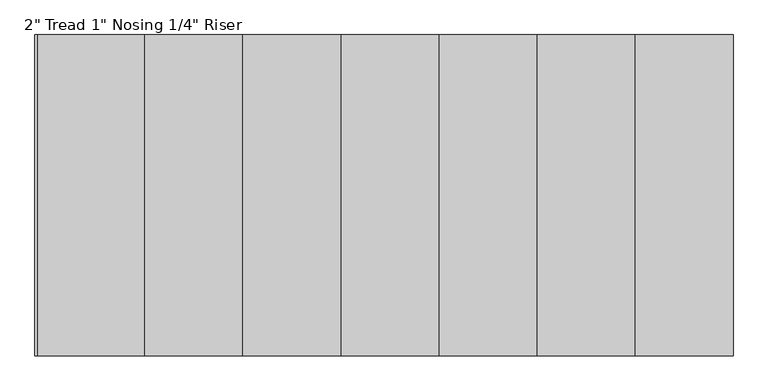
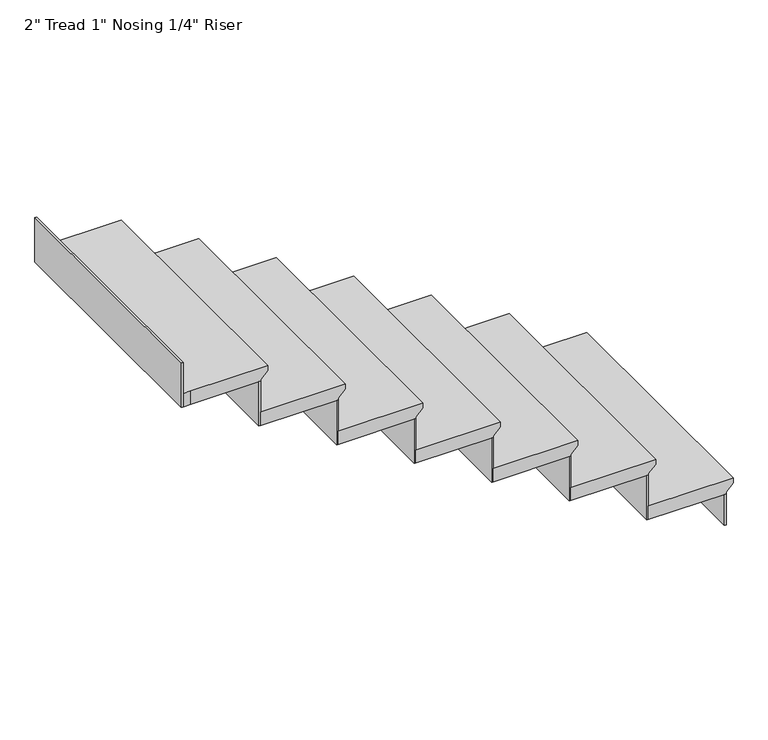
"""IFC4 building model written with IfcOpenShell, lengths in millimetres: stair flight geometry."""

from ifc_helpers import new_model, si_unit, origin, place, context, project, spatial, faceted_brep, source, transform, mapped, element, save


def stair_flight_13fda11b(model_context):
    return source(origin(), model_context, "Body", "Brep", [
        faceted_brep([(-12620.1777023, 559.4679075, 3503.0833333), (-12620.1777023, 559.4679075, 3522.1333333), (-12620.1777023, -354.9320925, 3522.1333333), (-12620.1777023, -354.9320925, 3503.0833333), (-12645.5777023, 559.4679075, 3477.6833333), (-12645.5777023, -354.9320925, 3477.6833333), (-12924.9777023, 559.4679075, 3522.1333333), (-12924.9777023, -354.9320925, 3522.1333333), (-12645.5777023, -354.9320925, 3471.3333333), (-12924.9777023, -354.9320925, 3471.3333333), (-12924.9777023, 559.4679075, 3471.3333333), (-12645.5777023, 559.4679075, 3471.3333333)], [[[0, 1, 2, 3]], [[4, 0, 3, 5]], [[2, 1, 6, 7]], [[8, 9, 10, 11]], [[2, 7, 9, 8, 5, 3]], [[8, 11, 4, 5]], [[6, 1, 0, 4, 11, 10]], [[7, 6, 10, 9]]]),
        faceted_brep([(-12645.5777023, 559.4679075, 3471.3333333), (-12645.5777023, 559.4679075, 3352.8), (-12651.9277023, 559.4679075, 3352.8), (-12651.9277023, 559.4679075, 3471.3333333), (-12645.5777023, -354.9320925, 3471.3333333), (-12651.9277023, -354.9320925, 3471.3333333), (-12651.9277023, -354.9320925, 3352.8), (-12645.5777023, -354.9320925, 3352.8)], [[[0, 1, 2, 3]], [[4, 5, 6, 7]], [[1, 0, 4, 7]], [[2, 1, 7, 6]], [[3, 2, 6, 5]], [[0, 3, 5, 4]]]),
        faceted_brep([(-12924.9777023, 559.4679075, 3640.6666667), (-12924.9777023, 559.4679075, 3471.3333333), (-12931.3277023, 559.4679075, 3471.3333333), (-12931.3277023, 559.4679075, 3640.6666667), (-12924.9777023, -354.9320925, 3640.6666667), (-12931.3277023, -354.9320925, 3640.6666667), (-12931.3277023, -354.9320925, 3471.3333333), (-12924.9777023, -354.9320925, 3471.3333333)], [[[0, 1, 2, 3]], [[4, 5, 6, 7]], [[1, 0, 4, 7]], [[2, 1, 7, 6]], [[3, 2, 6, 5]], [[0, 3, 5, 4]]]),
        faceted_brep([(-12899.5777023, -354.9320925, 3691.4666667), (-12899.5777023, 559.4679075, 3691.4666667), (-13204.3777023, 559.4679075, 3691.4666667), (-13204.3777023, -354.9320925, 3691.4666667), (-12924.9777023, -354.9320925, 3640.6666667), (-13204.3777023, -354.9320925, 3640.6666667), (-13204.3777023, 559.4679075, 3640.6666667), (-12924.9777023, 559.4679075, 3640.6666667), (-12924.9777023, -354.9320925, 3647.0166667), (-12899.5777023, -354.9320925, 3672.4166667), (-12924.9777023, 559.4679075, 3647.0166667), (-12899.5777023, 559.4679075, 3672.4166667)], [[[0, 1, 2, 3]], [[4, 5, 6, 7]], [[0, 3, 5, 4, 8, 9]], [[4, 7, 10, 8]], [[2, 1, 11, 10, 7, 6]], [[3, 2, 6, 5]], [[11, 1, 0, 9]], [[10, 11, 9, 8]]]),
        faceted_brep([(-13204.3777023, 559.4679075, 3810.0), (-13204.3777023, 559.4679075, 3640.6666667), (-13210.7277023, 559.4679075, 3640.6666667), (-13210.7277023, 559.4679075, 3810.0), (-13204.3777023, -354.9320925, 3810.0), (-13210.7277023, -354.9320925, 3810.0), (-13210.7277023, -354.9320925, 3640.6666667), (-13204.3777023, -354.9320925, 3640.6666667)], [[[0, 1, 2, 3]], [[4, 5, 6, 7]], [[1, 0, 4, 7]], [[2, 1, 7, 6]], [[3, 2, 6, 5]], [[0, 3, 5, 4]]]),
        faceted_brep([(-13178.9777023, -354.9320925, 3860.8), (-13178.9777023, 559.4679075, 3860.8), (-13483.7777023, 559.4679075, 3860.8), (-13483.7777023, -354.9320925, 3860.8), (-13204.3777023, -354.9320925, 3810.0), (-13483.7777023, -354.9320925, 3810.0), (-13483.7777023, 559.4679075, 3810.0), (-13204.3777023, 559.4679075, 3810.0), (-13204.3777023, -354.9320925, 3816.35), (-13178.9777023, -354.9320925, 3841.75), (-13204.3777023, 559.4679075, 3816.35), (-13178.9777023, 559.4679075, 3841.75)], [[[0, 1, 2, 3]], [[4, 5, 6, 7]], [[0, 3, 5, 4, 8, 9]], [[4, 7, 10, 8]], [[2, 1, 11, 10, 7, 6]], [[3, 2, 6, 5]], [[11, 1, 0, 9]], [[10, 11, 9, 8]]]),
        faceted_brep([(-13483.7777023, 559.4679075, 3979.3333333), (-13483.7777023, 559.4679075, 3810.0), (-13490.1277023, 559.4679075, 3810.0), (-13490.1277023, 559.4679075, 3979.3333333), (-13483.7777023, -354.9320925, 3979.3333333), (-13490.1277023, -354.9320925, 3979.3333333), (-13490.1277023, -354.9320925, 3810.0), (-13483.7777023, -354.9320925, 3810.0)], [[[0, 1, 2, 3]], [[4, 5, 6, 7]], [[1, 0, 4, 7]], [[2, 1, 7, 6]], [[3, 2, 6, 5]], [[0, 3, 5, 4]]]),
        faceted_brep([(-13458.3777023, -354.9320925, 4030.1333333), (-13458.3777023, 559.4679075, 4030.1333333), (-13763.1777023, 559.4679075, 4030.1333333), (-13763.1777023, -354.9320925, 4030.1333333), (-13483.7777023, -354.9320925, 3979.3333333), (-13763.1777023, -354.9320925, 3979.3333333), (-13763.1777023, 559.4679075, 3979.3333333), (-13483.7777023, 559.4679075, 3979.3333333), (-13483.7777023, -354.9320925, 3985.6833333), (-13458.3777023, -354.9320925, 4011.0833333), (-13483.7777023, 559.4679075, 3985.6833333), (-13458.3777023, 559.4679075, 4011.0833333)], [[[0, 1, 2, 3]], [[4, 5, 6, 7]], [[0, 3, 5, 4, 8, 9]], [[4, 7, 10, 8]], [[2, 1, 11, 10, 7, 6]], [[3, 2, 6, 5]], [[11, 1, 0, 9]], [[10, 11, 9, 8]]]),
        faceted_brep([(-13763.1777023, 559.4679075, 4148.6666667), (-13763.1777023, 559.4679075, 3979.3333333), (-13769.5277023, 559.4679075, 3979.3333333), (-13769.5277023, 559.4679075, 4148.6666667), (-13763.1777023, -354.9320925, 4148.6666667), (-13769.5277023, -354.9320925, 4148.6666667), (-13769.5277023, -354.9320925, 3979.3333333), (-13763.1777023, -354.9320925, 3979.3333333)], [[[0, 1, 2, 3]], [[4, 5, 6, 7]], [[1, 0, 4, 7]], [[2, 1, 7, 6]], [[3, 2, 6, 5]], [[0, 3, 5, 4]]]),
        faceted_brep([(-13737.7777023, -354.9320925, 4199.4666667), (-13737.7777023, 559.4679075, 4199.4666667), (-14042.5777023, 559.4679075, 4199.4666667), (-14042.5777023, -354.9320925, 4199.4666667), (-13763.1777023, -354.9320925, 4148.6666667), (-14042.5777023, -354.9320925, 4148.6666667), (-14042.5777023, 559.4679075, 4148.6666667), (-13763.1777023, 559.4679075, 4148.6666667), (-13763.1777023, -354.9320925, 4155.0166667), (-13737.7777023, -354.9320925, 4180.4166667), (-13763.1777023, 559.4679075, 4155.0166667), (-13737.7777023, 559.4679075, 4180.4166667)], [[[0, 1, 2, 3]], [[4, 5, 6, 7]], [[0, 3, 5, 4, 8, 9]], [[4, 7, 10, 8]], [[2, 1, 11, 10, 7, 6]], [[3, 2, 6, 5]], [[11, 1, 0, 9]], [[10, 11, 9, 8]]]),
        faceted_brep([(-14042.5777023, 559.4679075, 4318.0), (-14042.5777023, 559.4679075, 4148.6666667), (-14048.9277023, 559.4679075, 4148.6666667), (-14048.9277023, 559.4679075, 4318.0), (-14042.5777023, -354.9320925, 4318.0), (-14048.9277023, -354.9320925, 4318.0), (-14048.9277023, -354.9320925, 4148.6666667), (-14042.5777023, -354.9320925, 4148.6666667)], [[[0, 1, 2, 3]], [[4, 5, 6, 7]], [[1, 0, 4, 7]], [[2, 1, 7, 6]], [[3, 2, 6, 5]], [[0, 3, 5, 4]]]),
        faceted_brep([(-14017.1777023, -354.9320925, 4368.8), (-14017.1777023, 559.4679075, 4368.8), (-14321.9777023, 559.4679075, 4368.8), (-14321.9777023, -354.9320925, 4368.8), (-14042.5777023, -354.9320925, 4318.0), (-14321.9777023, -354.9320925, 4318.0), (-14321.9777023, 559.4679075, 4318.0), (-14042.5777023, 559.4679075, 4318.0), (-14042.5777023, -354.9320925, 4324.35), (-14017.1777023, -354.9320925, 4349.75), (-14042.5777023, 559.4679075, 4324.35), (-14017.1777023, 559.4679075, 4349.75)], [[[0, 1, 2, 3]], [[4, 5, 6, 7]], [[0, 3, 5, 4, 8, 9]], [[4, 7, 10, 8]], [[2, 1, 11, 10, 7, 6]], [[3, 2, 6, 5]], [[11, 1, 0, 9]], [[10, 11, 9, 8]]]),
        faceted_brep([(-14601.3777023, 559.4679075, 4656.6666667), (-14601.3777023, 559.4679075, 4487.3333333), (-14607.7277023, 559.4679075, 4487.3333333), (-14607.7277023, 559.4679075, 4656.6666667), (-14601.3777023, -354.9320925, 4656.6666667), (-14607.7277023, -354.9320925, 4656.6666667), (-14607.7277023, -354.9320925, 4487.3333333), (-14601.3777023, -354.9320925, 4487.3333333)], [[[0, 1, 2, 3]], [[4, 5, 6, 7]], [[1, 0, 4, 7]], [[2, 1, 7, 6]], [[3, 2, 6, 5]], [[0, 3, 5, 4]]]),
        faceted_brep([(-14321.9777023, 559.4679075, 4487.3333333), (-14321.9777023, 559.4679075, 4318.0), (-14328.3277023, 559.4679075, 4318.0), (-14328.3277023, 559.4679075, 4487.3333333), (-14321.9777023, -354.9320925, 4487.3333333), (-14328.3277023, -354.9320925, 4487.3333333), (-14328.3277023, -354.9320925, 4318.0), (-14321.9777023, -354.9320925, 4318.0)], [[[0, 1, 2, 3]], [[4, 5, 6, 7]], [[1, 0, 4, 7]], [[2, 1, 7, 6]], [[3, 2, 6, 5]], [[0, 3, 5, 4]]]),
        faceted_brep([(-14601.3777023, -354.9320925, 4538.1333333), (-14575.9777023, -354.9320925, 4538.1333333), (-14296.5777023, -354.9320925, 4538.1333333), (-14296.5777023, 559.4679075, 4538.1333333), (-14601.3777023, 559.4679075, 4538.1333333), (-14575.9777023, -354.9320925, 4487.3333333), (-14601.3777023, -354.9320925, 4487.3333333), (-14601.3777023, 559.4679075, 4487.3333333), (-14321.9777023, 559.4679075, 4487.3333333), (-14321.9777023, -354.9320925, 4487.3333333), (-14321.9777023, -354.9320925, 4493.6833333), (-14296.5777023, -354.9320925, 4519.0833333), (-14321.9777023, 559.4679075, 4493.6833333), (-14296.5777023, 559.4679075, 4519.0833333)], [[[0, 1, 2, 3, 4]], [[5, 6, 7, 8, 9]], [[1, 0, 6, 5]], [[2, 1, 5, 9, 10, 11]], [[9, 8, 12, 10]], [[4, 3, 13, 12, 8, 7]], [[0, 4, 7, 6]], [[13, 3, 2, 11]], [[12, 13, 11, 10]]]),
    ])


if __name__ == "__main__":
    model = new_model("IFC4")
    model_context = context("Model", 3, world=origin())
    ifc_project = project(units=[si_unit("LENGTHUNIT", "METRE", prefix="MILLI")], contexts=[model_context])
    site = spatial("IfcSite", under=ifc_project)
    building = spatial("IfcBuilding", under=site)
    placement = place(None, origin())
    stair_flight_shape = stair_flight_13fda11b(model_context)
    element("IfcStairFlight", 1, ObjectType="2\" Tread 1\" Nosing 1/4\" Riser", at=placement, inside=building, context=model_context, shape_type="MappedRepresentation", body=[
        mapped(stair_flight_shape, transform((0.0, 0.0, 0.0), x_axis=(1.0, 0.0, 0.0), y_axis=(0.0, 1.0, 0.0), z_axis=(0.0, 0.0, 1.0))),
    ])
    save(model, "model.ifc")
